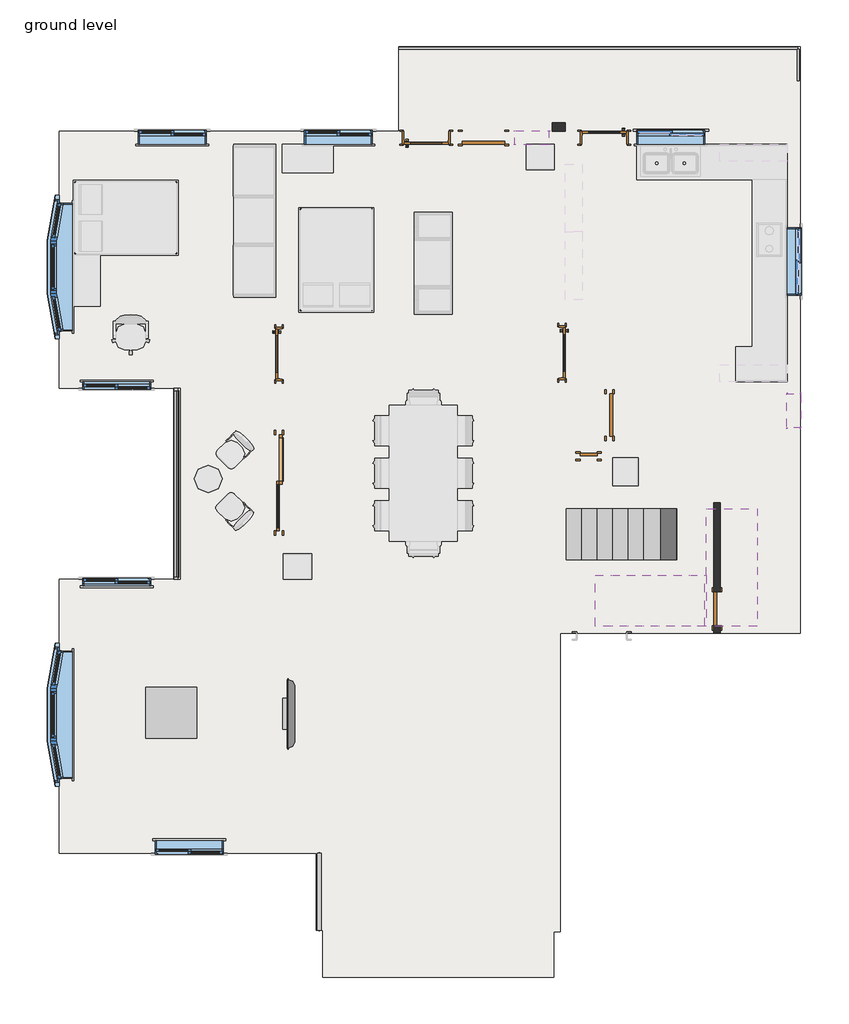
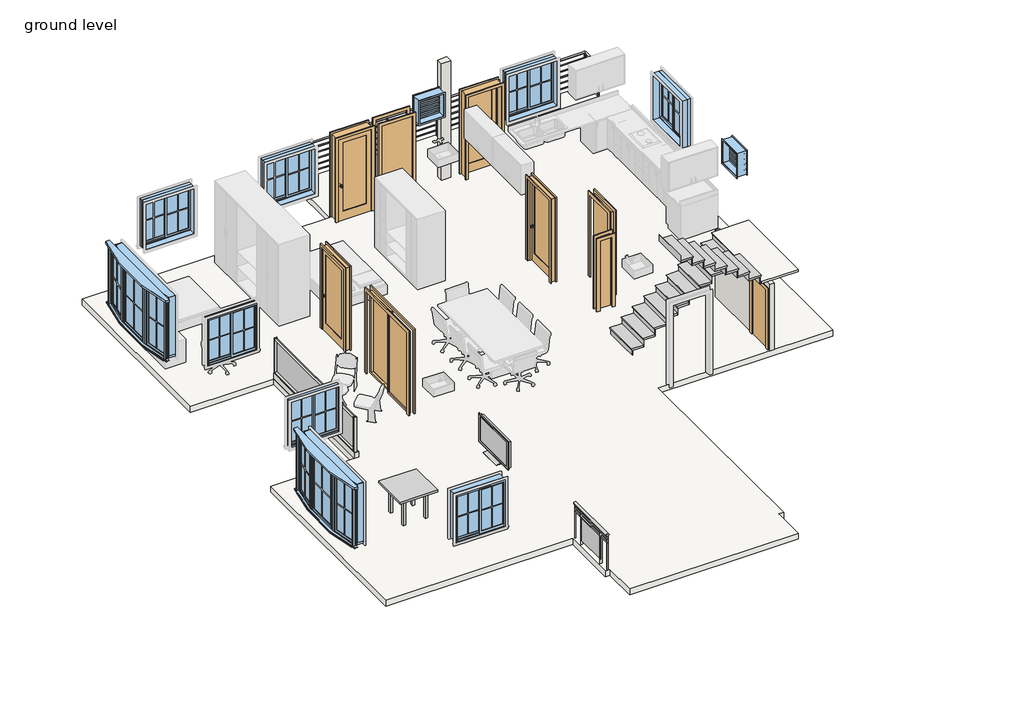
# One storey, part 1 of 2: 11 windows, 9 doors, 4 members, 3 railings, 3 walls, 2 furniture elements, 2 slabs, 2 stair flights, 1 plate.
"""IFC4 building model written with IfcOpenShell, lengths in millimetres."""

from ifc_helpers import new_model, si_unit, point, frame, frame_2d, origin, place, context, project, spatial, polyline, circle_curve, ellipse_curve, trimmed, segment, composite_curve, outline, extrude, transform, mapped, element, save
from ifc_brep_helpers import plane_surface, extruded_surface, advanced_brep
from components import door_505787c2, door_2631f38c, door_a3feeac7, door_3c6ab76a, door_b768bedd, door_bffbd567, door_78caadf7, door_bb98abfd, furniture_0b81fedb, furniture_5106913f, member_e759e848, member_235ee26f, member_c5b617ba, system_panel_glazed_59f99603, non_monolithic_landing_900e45c4, stair_flight_cfa64765, stair_flight_9d522be5, window_bf21e6cb, window_f2d8fef0, window_5af5dca6, window_ba0d9a6f

model = new_model("IFC4")

# Units and contexts
model_context = context("Model", 3, world=origin())
ifc_project = project(units=[si_unit("LENGTHUNIT", "METRE", prefix="MILLI")], contexts=[model_context])

# Site, building, storey
site = spatial("IfcSite", under=ifc_project)
building = spatial("IfcBuilding", under=site)
storey = spatial("IfcBuildingStorey", under=building, Name="ground level", Elevation=609.6)

# Doors
placement = place(None, origin())
door_shape = door_505787c2(model_context)
element("IfcDoor", 1, ObjectType="Door-Double-Sliding : 68\" x 84\"", at=placement, inside=storey, context=model_context, shape_type="MappedRepresentation", body=[
    mapped(door_shape, transform((-10169.8219122, 4291.3668074, 609.6), x_axis=(0.0, -1.0, 0.0), y_axis=(1.0, 0.0, 0.0), z_axis=(0.0, 0.0, 1.0))),
])
door_2_shape = door_2631f38c(model_context)
element("IfcDoor", 2, ObjectType="Door-Interior-Single-1_Panel-Wood : 32\" x 84\"", at=placement, inside=storey, context=model_context, shape_type="MappedRepresentation", body=[
    mapped(door_2_shape, transform((-7401.2219122, 10479.4418074, 609.6), x_axis=(1.0, 0.0, 0.0), y_axis=(0.0, 1.0, 0.0), z_axis=(0.0, 0.0, 1.0))),
])
element("IfcDoor", 3, ObjectType="Door-Interior-Single-1_Panel-Wood : 32\" x 84\"", at=placement, inside=storey, context=model_context, shape_type="MappedRepresentation", body=[
    mapped(door_2_shape, transform((-4203.9969122, 10485.7918074, 609.6), x_axis=(-1.0, 0.0, 0.0), y_axis=(0.0, -1.0, 0.0), z_axis=(0.0, 0.0, 1.0))),
])
door_3_shape = door_a3feeac7(model_context)
element("IfcDoor", 4, ObjectType="Door-Interior-Single-1_Panel-Wood : 36\" x 84\"", at=placement, inside=storey, context=model_context, shape_type="MappedRepresentation", body=[
    mapped(door_3_shape, transform((-10045.9969122, 6602.7668074, 609.6), x_axis=(0.0, -1.0, 0.0), y_axis=(1.0, 0.0, 0.0), z_axis=(0.0, 0.0, 1.0))),
])
door_4_shape = door_3c6ab76a(model_context)
element("IfcDoor", 5, ObjectType="Door-Interior-Single-1_Panel-Wood : 36\" x 84\"", at=placement, inside=storey, context=model_context, shape_type="MappedRepresentation", body=[
    mapped(door_4_shape, transform((-4962.8219122, 6624.9918074, 609.6), x_axis=(0.0, -1.0, 0.0), y_axis=(1.0, 0.0, 0.0), z_axis=(0.0, 0.0, 1.0))),
])
door_5_shape = door_b768bedd(model_context)
element("IfcDoor", 6, ObjectType="Single-Flush : 12\" x 72\"", at=placement, inside=storey, context=model_context, shape_type="MappedRepresentation", body=[
    mapped(door_5_shape, transform((-4486.5719122, 4767.6168074, 609.6), x_axis=(1.0, 0.0, 0.0), y_axis=(0.0, 1.0, 0.0), z_axis=(0.0, 0.0, 1.0))),
])
door_6_shape = door_bffbd567(model_context)
element("IfcDoor", 7, ObjectType="Single-Flush : 24\" x 60\"", at=placement, inside=storey, context=model_context, shape_type="MappedRepresentation", body=[
    mapped(door_6_shape, transform((-2180.7281622, 2027.5918074, 609.6), x_axis=(0.0, -1.0, 0.0), y_axis=(1.0, 0.0, 0.0), z_axis=(0.0, 0.0, 1.0))),
])
door_7_shape = door_78caadf7(model_context)
element("IfcDoor", 8, ObjectType="Single-Flush : 30\" x 84\"", at=placement, inside=storey, context=model_context, shape_type="MappedRepresentation", body=[
    mapped(door_7_shape, transform((-4111.9219122, 5504.2168074, 609.6), x_axis=(0.0, 1.0, 0.0), y_axis=(-1.0, 0.0, 0.0), z_axis=(0.0, 0.0, 1.0))),
])
door_8_shape = door_bb98abfd(model_context)
element("IfcDoor", 9, ObjectType="Single-Flush : 30\" x 84\"", at=placement, inside=storey, context=model_context, shape_type="MappedRepresentation", body=[
    mapped(door_8_shape, transform((-6372.5219122, 10482.6168074, 609.6), x_axis=(-1.0, 0.0, 0.0), y_axis=(0.0, -1.0, 0.0), z_axis=(0.0, 0.0, 1.0))),
])

# Furniture
furniture_shape = furniture_0b81fedb(model_context)
element("IfcFurniture", 10, ObjectType="TV - Flat Screen : 50\" 2", at=placement, inside=storey, context=model_context, shape_type="MappedRepresentation", body=[
    mapped(furniture_shape, transform((-9821.374617, 140.8722933, 1371.6), x_axis=(0.0, -1.0, 0.0), y_axis=(1.0, 0.0, 0.0), z_axis=(0.0, 0.0, 1.0))),
])
furniture_2_shape = furniture_5106913f(model_context)
element("IfcFurniture", 11, ObjectType="Table-Rectangular : 36\" x 36\"", at=placement, inside=storey, context=model_context, shape_type="MappedRepresentation", body=[
    mapped(furniture_2_shape, transform((-11973.2219122, 167.0418074, 609.6), x_axis=(1.0, 0.0, 0.0), y_axis=(0.0, 1.0, 0.0), z_axis=(0.0, 0.0, 1.0))),
])

# Members
member_shape = member_e759e848(model_context)
element("IfcMember", 12, ObjectType="Circular Mullion : 2.5\" Circular", at=placement, inside=storey, context=model_context, shape_type="MappedRepresentation", body=[
    mapped(member_shape, transform((-11890.6719122, 2595.9168074, 1676.4), x_axis=(0.0, 0.0, 1.0), y_axis=(-1.0, 0.0, 0.0), z_axis=(0.0, -1.0, 0.0))),
])
member_2_shape = member_235ee26f(model_context)
element("IfcMember", 13, ObjectType="Rectangular Mullion : 1.5\" x 2.5\" rectangular", at=placement, inside=storey, context=model_context, shape_type="MappedRepresentation", body=[
    mapped(member_2_shape, transform((-11890.6719122, 5947.562262, 762.0), x_axis=(0.0, 0.0, -1.0), y_axis=(-1.0, 0.0, 0.0), z_axis=(0.0, 1.0, 0.0))),
])
member_3_shape = member_c5b617ba(model_context)
element("IfcMember", 14, ObjectType="Rectangular Mullion : 1.5\" x 2.5\" rectangular", at=placement, inside=storey, context=model_context, shape_type="MappedRepresentation", body=[
    mapped(member_3_shape, transform((-11890.6719122, 5985.662262, 1676.4), x_axis=(0.0, 1.0, 0.0), y_axis=(-1.0, 0.0, 0.0), z_axis=(0.0, 0.0, 1.0))),
])
element("IfcMember", 15, ObjectType="Rectangular Mullion : 1.5\" x 2.5\" rectangular", at=placement, inside=storey, context=model_context, shape_type="MappedRepresentation", body=[
    mapped(member_3_shape, transform((-11890.6719122, 2557.8168074, 762.0), x_axis=(0.0, -1.0, 0.0), y_axis=(-1.0, 0.0, 0.0), z_axis=(0.0, 0.0, -1.0))),
])

# Plate
system_panel_glazed_shape = system_panel_glazed_59f99603(model_context)
element("IfcPlate", 16, ObjectType="System Panel : Glazed", at=placement, inside=storey, context=model_context, shape_type="MappedRepresentation", body=[
    mapped(system_panel_glazed_shape, transform((-11890.6719122, 4271.7395347, 800.1), x_axis=(0.0, -1.0, 0.0), y_axis=(1.0, 0.0, 0.0), z_axis=(0.0, 0.0, 1.0))),
])

# Railings
element("IfcRailing", 17, ObjectType="Glass Panel - Bottom Fill", at=placement, inside=storey, context=model_context, shape_type="SolidModel", body=[
    advanced_brep(
    [(-9357.0219122, -3741.3831926, 1524.0), (-9280.8219122, -3741.3831926, 1524.0), (-9357.0219122, -2357.0831926, 1524.0), (-9280.8219122, -2357.0831926, 1524.0)],
    [
        (0, 1, ellipse_curve(frame((-9318.9219122, -3741.3831926, 1524.0), z_axis=(0.0, -1.0, 0.0), x_axis=(1.0, 0.0, 0.0)), 38.1, 28.575)),
        (1, 0, ellipse_curve(frame((-9318.9219122, -3741.3831926, 1524.0), z_axis=(0.0, -1.0, 0.0), x_axis=(1.0, 0.0, 0.0)), 38.1, 28.575)),
        (2, 3, ellipse_curve(frame((-9318.9219122, -2357.0831926, 1524.0), z_axis=(0.0, 1.0, 0.0), x_axis=(1.0, 0.0, 0.0)), 38.1, 28.575)),
        (3, 2, ellipse_curve(frame((-9318.9219122, -2357.0831926, 1524.0), z_axis=(0.0, 1.0, 0.0), x_axis=(1.0, 0.0, 0.0)), 38.1, 28.575)),
        (0, 2),
        (3, 1),
    ],
    [
        plane_surface(frame((-9318.9219122, -3741.3831926, 1524.0), z_axis=(0.0, -1.0, 0.0), x_axis=(0.0, 0.0, 1.0))),
        plane_surface(frame((-9318.9219122, -2357.0831926, 1524.0), z_axis=(0.0, 1.0, 0.0), x_axis=(0.0, 0.0, 1.0))),
        extruded_surface(trimmed(ellipse_curve(frame((-9318.9219122, -2357.0831926, 1524.0), z_axis=(0.0, -1.0, 0.0), x_axis=(1.0, 0.0, 0.0)), 38.1, 28.575), [point((-9357.0219122, -2357.0831926, 1524.0))], [point((-9280.8219122, -2357.0831926, 1524.0))], True, "CARTESIAN"), (0.0, -1384.2999999999997, 0.0), 1384.2999999999997),
        extruded_surface(trimmed(ellipse_curve(frame((-9318.9219122, -2357.0831926, 1524.0), z_axis=(0.0, -1.0, 0.0), x_axis=(1.0, 0.0, 0.0)), 38.1, 28.575), [point((-9280.8219122, -2357.0831926, 1524.0))], [point((-9357.0219122, -2357.0831926, 1524.0))], True, "CARTESIAN"), (0.0, -1384.2999999999997, 0.0), 1384.2999999999997),
    ],
    [
        (0, [[1, 2]]),
        (1, [[3, 4]]),
        (2, [[-1, 5, -4, 6]]),
        (3, [[-2, -6, -3, -5]]),
    ],
),
    extrude(outline(polyline([(-9306.2219122, -3741.3831926), (-9331.6219122, -3741.3831926), (-9331.6219122, -2357.0831926), (-9306.2219122, -2357.0831926), (-9306.2219122, -3741.3831926)])), frame((0.0, 0.0, 1409.7), z_axis=(0.0, 0.0, 1.0), x_axis=(1.0, 0.0, 0.0)), (0.0, 0.0, 1.0), 25.4),
    extrude(outline(polyline([(-9306.2219122, -3741.3831926), (-9331.6219122, -3741.3831926), (-9331.6219122, -2357.0831926), (-9306.2219122, -2357.0831926), (-9306.2219122, -3741.3831926)])), frame((0.0, 0.0, 1308.1), z_axis=(0.0, 0.0, 1.0), x_axis=(1.0, 0.0, 0.0)), (0.0, 0.0, 1.0), 25.4),
    extrude(outline(polyline([(-9293.5219122, -2649.1831926), (-9344.3219122, -2649.1831926), (-9344.3219122, -2636.4831926), (-9293.5219122, -2636.4831926), (-9293.5219122, -2649.1831926)])), frame((0.0, 0.0, 609.6), z_axis=(0.0, 0.0, 1.0), x_axis=(1.0, 0.0, 0.0)), (0.0, 0.0, 1.0), 885.825),
    extrude(outline(polyline([(-9325.4570692, -3455.6331926), (-9325.4570692, -2642.8331926), (-9319.1070692, -2642.8331926), (-9319.1070692, -3455.6331926), (-9325.4570692, -3455.6331926)])), frame((0.0, 0.0, 711.2), z_axis=(0.0, 0.0, 1.0), x_axis=(1.0, 0.0, 0.0)), (0.0, 0.0, 1.0), 596.9),
    extrude(outline(polyline([(-9293.5219122, -3461.9831926), (-9344.3219122, -3461.9831926), (-9344.3219122, -3449.2831926), (-9293.5219122, -3449.2831926), (-9293.5219122, -3461.9831926)])), frame((0.0, 0.0, 609.6), z_axis=(0.0, 0.0, 1.0), x_axis=(1.0, 0.0, 0.0)), (0.0, 0.0, 1.0), 885.825),
    extrude(outline(polyline([(-9309.3969122, -2369.7831926), (-9328.4469122, -2369.7831926), (-9328.4469122, -2350.7331926), (-9309.3969122, -2350.7331926), (-9309.3969122, -2369.7831926)])), frame((0.0, 0.0, 609.6), z_axis=(0.0, 0.0, 1.0), x_axis=(1.0, 0.0, 0.0)), (0.0, 0.0, 1.0), 885.825),
    extrude(outline(polyline([(-9309.3969122, -3747.7331926), (-9328.4469122, -3747.7331926), (-9328.4469122, -3728.6831926), (-9309.3969122, -3728.6831926), (-9309.3969122, -3747.7331926)])), frame((0.0, 0.0, 609.6), z_axis=(0.0, 0.0, 1.0), x_axis=(1.0, 0.0, 0.0)), (0.0, 0.0, 1.0), 885.825),
])
element("IfcRailing", 18, ObjectType="Handrail - Pipe", at=placement, inside=storey, context=model_context, shape_type="SweptSolid", body=[
    extrude(outline(composite_curve([segment(trimmed(circle_curve(frame_2d((1504.95, -727.3719122)), 19.05), [point((1504.95, -708.3219122))], [point((1504.95, -746.4219122))], False, "CARTESIAN"), True, "CONTINUOUS"), segment(trimmed(circle_curve(frame_2d((1504.95, -727.3719122)), 19.05), [point((1504.95, -746.4219122))], [point((1504.95, -708.3219122))], False, "CARTESIAN"), True, "CONTINUOUS")], self_intersect=False)), frame((0.0, 11511.3168074, 0.0), z_axis=(0.0, 1.0, 0.0), x_axis=(0.0, 0.0, 1.0)), (0.0, 0.0, 1.0), 558.8),
    extrude(outline(composite_curve([segment(trimmed(circle_curve(frame_2d((1358.9, -727.3719122)), 12.7), [point((1358.9, -740.0719122))], [point((1358.9, -714.6719122))], False, "CARTESIAN"), True, "CONTINUOUS"), segment(trimmed(circle_curve(frame_2d((1358.9, -727.3719122)), 12.7), [point((1358.9, -714.6719122))], [point((1358.9, -740.0719122))], False, "CARTESIAN"), True, "CONTINUOUS")], self_intersect=False)), frame((0.0, 11511.3168074, 0.0), z_axis=(0.0, 1.0, 0.0), x_axis=(0.0, 0.0, 1.0)), (0.0, 0.0, 1.0), 558.8),
    extrude(outline(composite_curve([segment(trimmed(circle_curve(frame_2d((1206.5, -727.3719122)), 12.7), [point((1206.5, -740.0719122))], [point((1206.5, -714.6719122))], False, "CARTESIAN"), True, "CONTINUOUS"), segment(trimmed(circle_curve(frame_2d((1206.5, -727.3719122)), 12.7), [point((1206.5, -714.6719122))], [point((1206.5, -740.0719122))], False, "CARTESIAN"), True, "CONTINUOUS")], self_intersect=False)), frame((0.0, 11511.3168074, 0.0), z_axis=(0.0, 1.0, 0.0), x_axis=(0.0, 0.0, 1.0)), (0.0, 0.0, 1.0), 558.8),
    extrude(outline(composite_curve([segment(trimmed(circle_curve(frame_2d((1054.1, -727.3719122)), 12.7), [point((1054.1, -740.0719122))], [point((1054.1, -714.6719122))], False, "CARTESIAN"), True, "CONTINUOUS"), segment(trimmed(circle_curve(frame_2d((1054.1, -727.3719122)), 12.7), [point((1054.1, -714.6719122))], [point((1054.1, -740.0719122))], False, "CARTESIAN"), True, "CONTINUOUS")], self_intersect=False)), frame((0.0, 11511.3168074, 0.0), z_axis=(0.0, 1.0, 0.0), x_axis=(0.0, 0.0, 1.0)), (0.0, 0.0, 1.0), 558.8),
    extrude(outline(composite_curve([segment(trimmed(circle_curve(frame_2d((901.7, -727.3719122)), 12.7), [point((901.7, -740.0719122))], [point((901.7, -714.6719122))], False, "CARTESIAN"), True, "CONTINUOUS"), segment(trimmed(circle_curve(frame_2d((901.7, -727.3719122)), 12.7), [point((901.7, -714.6719122))], [point((901.7, -740.0719122))], False, "CARTESIAN"), True, "CONTINUOUS")], self_intersect=False)), frame((0.0, 11511.3168074, 0.0), z_axis=(0.0, 1.0, 0.0), x_axis=(0.0, 0.0, 1.0)), (0.0, 0.0, 1.0), 558.8),
    extrude(outline(composite_curve([segment(trimmed(circle_curve(frame_2d((749.3, -727.3719122)), 12.7), [point((749.3, -740.0719122))], [point((749.3, -714.6719122))], False, "CARTESIAN"), True, "CONTINUOUS"), segment(trimmed(circle_curve(frame_2d((749.3, -727.3719122)), 12.7), [point((749.3, -714.6719122))], [point((749.3, -740.0719122))], False, "CARTESIAN"), True, "CONTINUOUS")], self_intersect=False)), frame((0.0, 11511.3168074, 0.0), z_axis=(0.0, 1.0, 0.0), x_axis=(0.0, 0.0, 1.0)), (0.0, 0.0, 1.0), 558.8),
    extrude(outline(composite_curve([segment(trimmed(circle_curve(frame_2d((-727.3719122, 12057.4168074)), 12.7), [point((-740.0719122, 12057.4168074))], [point((-714.6719122, 12057.4168074))], False, "CARTESIAN"), True, "CONTINUOUS"), segment(trimmed(circle_curve(frame_2d((-727.3719122, 12057.4168074)), 12.7), [point((-714.6719122, 12057.4168074))], [point((-740.0719122, 12057.4168074))], False, "CARTESIAN"), True, "CONTINUOUS")], self_intersect=False)), frame((0.0, 0.0, 609.6), z_axis=(0.0, 0.0, 1.0), x_axis=(1.0, 0.0, 0.0)), (0.0, 0.0, 1.0), 876.3),
    extrude(outline(composite_curve([segment(trimmed(circle_curve(frame_2d((-727.3719122, 11524.0168074)), 12.7), [point((-740.0719122, 11524.0168074))], [point((-714.6719122, 11524.0168074))], False, "CARTESIAN"), True, "CONTINUOUS"), segment(trimmed(circle_curve(frame_2d((-727.3719122, 11524.0168074)), 12.7), [point((-714.6719122, 11524.0168074))], [point((-740.0719122, 11524.0168074))], False, "CARTESIAN"), True, "CONTINUOUS")], self_intersect=False)), frame((0.0, 0.0, 609.6), z_axis=(0.0, 0.0, 1.0), x_axis=(1.0, 0.0, 0.0)), (0.0, 0.0, 1.0), 876.3),
])
element("IfcRailing", 19, ObjectType="Handrail - Pipe", at=placement, inside=storey, context=model_context, shape_type="SweptSolid", body=[
    extrude(outline(composite_curve([segment(trimmed(circle_curve(frame_2d((12090.8688347, 1504.95)), 19.05), [point((12109.9188347, 1504.95))], [point((12071.8188347, 1504.95))], False, "CARTESIAN"), True, "CONTINUOUS"), segment(trimmed(circle_curve(frame_2d((12090.8688347, 1504.95)), 19.05), [point((12071.8188347, 1504.95))], [point((12109.9188347, 1504.95))], False, "CARTESIAN"), True, "CONTINUOUS")], self_intersect=False)), frame((-7890.1719122, 0.0, 0.0), z_axis=(1.0, 0.0, 0.0), x_axis=(0.0, 1.0, 0.0)), (0.0, 0.0, 1.0), 7160.6305666),
    extrude(outline(composite_curve([segment(trimmed(circle_curve(frame_2d((12090.8688347, 1358.9)), 12.7), [point((12078.1688347, 1358.9))], [point((12103.5688347, 1358.9))], False, "CARTESIAN"), True, "CONTINUOUS"), segment(trimmed(circle_curve(frame_2d((12090.8688347, 1358.9)), 12.7), [point((12103.5688347, 1358.9))], [point((12078.1688347, 1358.9))], False, "CARTESIAN"), True, "CONTINUOUS")], self_intersect=False)), frame((-7890.1719122, 0.0, 0.0), z_axis=(1.0, 0.0, 0.0), x_axis=(0.0, 1.0, 0.0)), (0.0, 0.0, 1.0), 7160.6305666),
    extrude(outline(composite_curve([segment(trimmed(circle_curve(frame_2d((12090.8688347, 1206.5)), 12.7), [point((12078.1688347, 1206.5))], [point((12103.5688347, 1206.5))], False, "CARTESIAN"), True, "CONTINUOUS"), segment(trimmed(circle_curve(frame_2d((12090.8688347, 1206.5)), 12.7), [point((12103.5688347, 1206.5))], [point((12078.1688347, 1206.5))], False, "CARTESIAN"), True, "CONTINUOUS")], self_intersect=False)), frame((-7890.1719122, 0.0, 0.0), z_axis=(1.0, 0.0, 0.0), x_axis=(0.0, 1.0, 0.0)), (0.0, 0.0, 1.0), 7160.6305666),
    extrude(outline(composite_curve([segment(trimmed(circle_curve(frame_2d((12090.8688347, 1054.1)), 12.7), [point((12078.1688347, 1054.1))], [point((12103.5688347, 1054.1))], False, "CARTESIAN"), True, "CONTINUOUS"), segment(trimmed(circle_curve(frame_2d((12090.8688347, 1054.1)), 12.7), [point((12103.5688347, 1054.1))], [point((12078.1688347, 1054.1))], False, "CARTESIAN"), True, "CONTINUOUS")], self_intersect=False)), frame((-7890.1719122, 0.0, 0.0), z_axis=(1.0, 0.0, 0.0), x_axis=(0.0, 1.0, 0.0)), (0.0, 0.0, 1.0), 7160.6305666),
    extrude(outline(composite_curve([segment(trimmed(circle_curve(frame_2d((12090.8688347, 901.7)), 12.7), [point((12078.1688347, 901.7))], [point((12103.5688347, 901.7))], False, "CARTESIAN"), True, "CONTINUOUS"), segment(trimmed(circle_curve(frame_2d((12090.8688347, 901.7)), 12.7), [point((12103.5688347, 901.7))], [point((12078.1688347, 901.7))], False, "CARTESIAN"), True, "CONTINUOUS")], self_intersect=False)), frame((-7890.1719122, 0.0, 0.0), z_axis=(1.0, 0.0, 0.0), x_axis=(0.0, 1.0, 0.0)), (0.0, 0.0, 1.0), 7160.6305666),
    extrude(outline(composite_curve([segment(trimmed(circle_curve(frame_2d((12090.8688347, 749.3)), 12.7), [point((12078.1688347, 749.3))], [point((12103.5688347, 749.3))], False, "CARTESIAN"), True, "CONTINUOUS"), segment(trimmed(circle_curve(frame_2d((12090.8688347, 749.3)), 12.7), [point((12103.5688347, 749.3))], [point((12078.1688347, 749.3))], False, "CARTESIAN"), True, "CONTINUOUS")], self_intersect=False)), frame((-7890.1719122, 0.0, 0.0), z_axis=(1.0, 0.0, 0.0), x_axis=(0.0, 1.0, 0.0)), (0.0, 0.0, 1.0), 7160.6305666),
    extrude(outline(composite_curve([segment(trimmed(circle_curve(frame_2d((-6825.5413455, 12090.8688347)), 12.7), [point((-6825.5413455, 12078.1688347))], [point((-6825.5413455, 12103.5688347))], False, "CARTESIAN"), True, "CONTINUOUS"), segment(trimmed(circle_curve(frame_2d((-6825.5413455, 12090.8688347)), 12.7), [point((-6825.5413455, 12103.5688347))], [point((-6825.5413455, 12078.1688347))], False, "CARTESIAN"), True, "CONTINUOUS")], self_intersect=False)), frame((0.0, 0.0, 609.6), z_axis=(0.0, 0.0, 1.0), x_axis=(1.0, 0.0, 0.0)), (0.0, 0.0, 1.0), 876.3),
    extrude(outline(composite_curve([segment(trimmed(circle_curve(frame_2d((-5606.3413455, 12090.8688347)), 12.7), [point((-5606.3413455, 12078.1688347))], [point((-5606.3413455, 12103.5688347))], False, "CARTESIAN"), True, "CONTINUOUS"), segment(trimmed(circle_curve(frame_2d((-5606.3413455, 12090.8688347)), 12.7), [point((-5606.3413455, 12103.5688347))], [point((-5606.3413455, 12078.1688347))], False, "CARTESIAN"), True, "CONTINUOUS")], self_intersect=False)), frame((0.0, 0.0, 609.6), z_axis=(0.0, 0.0, 1.0), x_axis=(1.0, 0.0, 0.0)), (0.0, 0.0, 1.0), 876.3),
    extrude(outline(composite_curve([segment(trimmed(circle_curve(frame_2d((-4387.1413455, 12090.8688347)), 12.7), [point((-4387.1413455, 12078.1688347))], [point((-4387.1413455, 12103.5688347))], False, "CARTESIAN"), True, "CONTINUOUS"), segment(trimmed(circle_curve(frame_2d((-4387.1413455, 12090.8688347)), 12.7), [point((-4387.1413455, 12103.5688347))], [point((-4387.1413455, 12078.1688347))], False, "CARTESIAN"), True, "CONTINUOUS")], self_intersect=False)), frame((0.0, 0.0, 609.6), z_axis=(0.0, 0.0, 1.0), x_axis=(1.0, 0.0, 0.0)), (0.0, 0.0, 1.0), 876.3),
    extrude(outline(composite_curve([segment(trimmed(circle_curve(frame_2d((-3167.9413455, 12090.8688347)), 12.7), [point((-3167.9413455, 12078.1688347))], [point((-3167.9413455, 12103.5688347))], False, "CARTESIAN"), True, "CONTINUOUS"), segment(trimmed(circle_curve(frame_2d((-3167.9413455, 12090.8688347)), 12.7), [point((-3167.9413455, 12103.5688347))], [point((-3167.9413455, 12078.1688347))], False, "CARTESIAN"), True, "CONTINUOUS")], self_intersect=False)), frame((0.0, 0.0, 609.6), z_axis=(0.0, 0.0, 1.0), x_axis=(1.0, 0.0, 0.0)), (0.0, 0.0, 1.0), 876.3),
    extrude(outline(composite_curve([segment(trimmed(circle_curve(frame_2d((-1948.7413455, 12090.8688347)), 12.7), [point((-1948.7413455, 12078.1688347))], [point((-1948.7413455, 12103.5688347))], False, "CARTESIAN"), True, "CONTINUOUS"), segment(trimmed(circle_curve(frame_2d((-1948.7413455, 12090.8688347)), 12.7), [point((-1948.7413455, 12103.5688347))], [point((-1948.7413455, 12078.1688347))], False, "CARTESIAN"), True, "CONTINUOUS")], self_intersect=False)), frame((0.0, 0.0, 609.6), z_axis=(0.0, 0.0, 1.0), x_axis=(1.0, 0.0, 0.0)), (0.0, 0.0, 1.0), 876.3),
    extrude(outline(composite_curve([segment(trimmed(circle_curve(frame_2d((-7877.4719122, 12090.8688347)), 12.7), [point((-7877.4719122, 12078.1688347))], [point((-7877.4719122, 12103.5688347))], False, "CARTESIAN"), True, "CONTINUOUS"), segment(trimmed(circle_curve(frame_2d((-7877.4719122, 12090.8688347)), 12.7), [point((-7877.4719122, 12103.5688347))], [point((-7877.4719122, 12078.1688347))], False, "CARTESIAN"), True, "CONTINUOUS")], self_intersect=False)), frame((0.0, 0.0, 609.6), z_axis=(0.0, 0.0, 1.0), x_axis=(1.0, 0.0, 0.0)), (0.0, 0.0, 1.0), 876.3),
    extrude(outline(composite_curve([segment(trimmed(circle_curve(frame_2d((-742.2413455, 12090.8688347)), 12.7), [point((-742.2413455, 12078.1688347))], [point((-742.2413455, 12103.5688347))], False, "CARTESIAN"), True, "CONTINUOUS"), segment(trimmed(circle_curve(frame_2d((-742.2413455, 12090.8688347)), 12.7), [point((-742.2413455, 12103.5688347))], [point((-742.2413455, 12078.1688347))], False, "CARTESIAN"), True, "CONTINUOUS")], self_intersect=False)), frame((0.0, 0.0, 609.6), z_axis=(0.0, 0.0, 1.0), x_axis=(1.0, 0.0, 0.0)), (0.0, 0.0, 1.0), 876.3),
])

# Slabs
element("IfcSlab", 20, ObjectType="Generic - 6\"", at=placement, inside=storey, context=model_context, shape_type="SweptSolid", body=[
    extrude(outline(polyline([(-7890.1719122, 10596.9168074), (-7890.1719122, 12120.9168074), (-689.2719122, 12120.9168074), (-689.2719122, 1595.7918074), (-4994.5719122, 1595.7918074), (-4994.5719122, -2357.0831926), (-4993.7781622, -2357.0831926), (-4993.7781622, -3766.7831926), (-5108.0781622, -3766.7831926), (-5108.0781622, -4585.9331926), (-9261.7719122, -4585.9331926), (-9261.7719122, -3741.3831926), (-9376.0719122, -3741.3831926), (-9376.0719122, -2357.0831926), (-13986.1719122, -2357.0831926), (-13986.1719122, 2557.8168074), (-11928.7719122, 2557.8168074), (-11928.7719122, 5985.662262), (-13986.1719122, 5985.662262), (-13986.1719122, 10596.9168074), (-7890.1719122, 10596.9168074)])), frame((0.0, 0.0, 457.2), z_axis=(0.0, 0.0, 1.0), x_axis=(1.0, 0.0, 0.0)), (0.0, 0.0, 1.0), 152.4),
])
non_monolithic_landing_shape = non_monolithic_landing_900e45c4(model_context)
element("IfcSlab", 21, ObjectType="Non-Monolithic Landing", at=placement, inside=storey, context=model_context, shape_type="MappedRepresentation", body=[
    mapped(non_monolithic_landing_shape, transform((0.0, 0.0, 0.0), x_axis=(1.0, 0.0, 0.0), y_axis=(0.0, 1.0, 0.0), z_axis=(0.0, 0.0, 1.0))),
])

# Stair flights
stair_flight_shape = stair_flight_cfa64765(model_context)
element("IfcStairFlight", 22, ObjectType="2\" Tread 1\" Nosing 1/4\" Riser", at=placement, inside=storey, context=model_context, shape_type="MappedRepresentation", body=[
    mapped(stair_flight_shape, transform((0.0, 0.0, 0.0), x_axis=(1.0, 0.0, 0.0), y_axis=(0.0, 1.0, 0.0), z_axis=(0.0, 0.0, 1.0))),
])
stair_flight_2_shape = stair_flight_9d522be5(model_context)
element("IfcStairFlight", 23, ObjectType="2\" Tread 1\" Nosing 1/4\" Riser", at=placement, inside=storey, context=model_context, shape_type="MappedRepresentation", body=[
    mapped(stair_flight_2_shape, transform((0.0, 0.0, 0.0), x_axis=(1.0, 0.0, 0.0), y_axis=(0.0, 1.0, 0.0), z_axis=(0.0, 0.0, 1.0))),
])

# Walls
element("IfcWall", 24, ObjectType="Generic - 4.5\"", at=placement, inside=storey, context=model_context, shape_type="SweptSolid", body=[
    extrude(outline(polyline([(1722.7918074, 2133.6), (1722.7918074, 609.6), (1595.7918074, 609.6), (1595.7918074, 2336.8), (3929.4168074, 2336.8), (3929.4168074, 609.6), (2332.3918074, 609.6), (2332.3918074, 2133.6), (1722.7918074, 2133.6)])), frame((-2237.8781622, 0.0, 0.0), z_axis=(1.0, 0.0, 0.0), x_axis=(0.0, 1.0, 0.0)), (0.0, 0.0, 1.0), 114.3),
])
element("IfcWall", 25, ObjectType="Generic - 4.5\"", at=placement, inside=storey, context=model_context, shape_type="SweptSolid", body=[
    extrude(outline(polyline([(-11928.7719122, 2557.8168074), (-11928.7719122, 5985.662262), (-11814.4719122, 5985.662262), (-11814.4719122, 2557.8168074), (-11928.7719122, 2557.8168074)])), frame((0.0, 0.0, 609.6), z_axis=(0.0, 0.0, 1.0), x_axis=(1.0, 0.0, 0.0)), (0.0, 0.0, 1.0), 152.4),
])
element("IfcWall", 26, ObjectType="Generic - 9\"", at=placement, inside=storey, context=model_context, shape_type="SweptSolid", body=[
    extrude(outline(polyline([(-4908.8469122, 10749.3168074), (-4908.8469122, 10596.9168074), (-5137.4469122, 10596.9168074), (-5137.4469122, 10749.3168074), (-4908.8469122, 10749.3168074)])), frame((0.0, 0.0, 609.6), z_axis=(0.0, 0.0, 1.0), x_axis=(1.0, 0.0, 0.0)), (0.0, 0.0, 1.0), 3048.0),
])

# Windows
window_shape = window_bf21e6cb(model_context)
element("IfcWindow", 27, ObjectType="Window-Bay-Casement-10_Degree_Angle : 90\" x 60\" x 6\"", at=placement, inside=storey, context=model_context, shape_type="MappedRepresentation", body=[
    mapped(window_shape, transform((-13871.8719122, 8161.6918074, 609.6), x_axis=(0.0, 1.0, 0.0), y_axis=(-1.0, 0.0, 0.0), z_axis=(0.0, 0.0, 1.0))),
])
element("IfcWindow", 28, ObjectType="Window-Bay-Casement-10_Degree_Angle : 90\" x 60\" x 6\"", at=placement, inside=storey, context=model_context, shape_type="MappedRepresentation", body=[
    mapped(window_shape, transform((-13871.8719122, 128.9418074, 609.6), x_axis=(0.0, 1.0, 0.0), y_axis=(-1.0, 0.0, 0.0), z_axis=(0.0, 0.0, 1.0))),
])
window_2_shape = window_f2d8fef0(model_context)
element("IfcWindow", 29, ObjectType="Window-Louvers : 24\" x 24\"", at=placement, inside=storey, context=model_context, shape_type="MappedRepresentation", body=[
    mapped(window_2_shape, transform((-5505.7469122, 10488.9668074, 1524.0), x_axis=(1.0, 0.0, 0.0), y_axis=(0.0, 1.0, 0.0), z_axis=(0.0, 0.0, 1.0))),
])
element("IfcWindow", 30, ObjectType="Window-Louvers : 24\" x 24\"", at=placement, inside=storey, context=model_context, shape_type="MappedRepresentation", body=[
    mapped(window_2_shape, transform((-797.2219122, 5586.7668074, 1524.0), x_axis=(0.0, -1.0, 0.0), y_axis=(1.0, 0.0, 0.0), z_axis=(0.0, 0.0, 1.0))),
])
window_3_shape = window_5af5dca6(model_context)
element("IfcWindow", 31, ObjectType="Window-Sliding-Double : 48\" x 48\"", at=placement, inside=storey, context=model_context, shape_type="MappedRepresentation", body=[
    mapped(window_3_shape, transform((-11652.5469122, -2246.5931926, 609.6), x_axis=(-1.0, 0.0, 0.0), y_axis=(0.0, -1.0, 0.0), z_axis=(0.0, 0.0, 1.0))),
])
element("IfcWindow", 32, ObjectType="Window-Sliding-Double : 48\" x 48\"", at=placement, inside=storey, context=model_context, shape_type="MappedRepresentation", body=[
    mapped(window_3_shape, transform((-799.7619122, 8263.2918074, 838.2), x_axis=(0.0, -1.0, 0.0), y_axis=(1.0, 0.0, 0.0), z_axis=(0.0, 0.0, 1.0))),
])
element("IfcWindow", 33, ObjectType="Window-Sliding-Double : 48\" x 48\"", at=placement, inside=storey, context=model_context, shape_type="MappedRepresentation", body=[
    mapped(window_3_shape, transform((-8976.0219122, 10486.4268074, 609.6), x_axis=(1.0, 0.0, 0.0), y_axis=(0.0, 1.0, 0.0), z_axis=(0.0, 0.0, 1.0))),
])
element("IfcWindow", 34, ObjectType="Window-Sliding-Double : 48\" x 48\"", at=placement, inside=storey, context=model_context, shape_type="MappedRepresentation", body=[
    mapped(window_3_shape, transform((-11957.3469122, 10486.4268074, 609.6), x_axis=(1.0, 0.0, 0.0), y_axis=(0.0, 1.0, 0.0), z_axis=(0.0, 0.0, 1.0))),
])
element("IfcWindow", 35, ObjectType="Window-Sliding-Double : 48\" x 48\"", at=placement, inside=storey, context=model_context, shape_type="MappedRepresentation", body=[
    mapped(window_3_shape, transform((-3010.1969122, 10486.4268074, 812.8), x_axis=(1.0, 0.0, 0.0), y_axis=(0.0, 1.0, 0.0), z_axis=(0.0, 0.0, 1.0))),
])
window_4_shape = window_ba0d9a6f(model_context)
element("IfcWindow", 36, ObjectType="Window-Sliding-Double : 48\" x 48\"", at=placement, inside=storey, context=model_context, shape_type="MappedRepresentation", body=[
    mapped(window_4_shape, transform((-12957.4719122, 2504.4768074, 609.6), x_axis=(1.0, 0.0, 0.0), y_axis=(0.0, 1.0, 0.0), z_axis=(0.0, 0.0, 1.0))),
])
element("IfcWindow", 37, ObjectType="Window-Sliding-Double : 48\" x 48\"", at=placement, inside=storey, context=model_context, shape_type="MappedRepresentation", body=[
    mapped(window_4_shape, transform((-12957.4719122, 6040.1568074, 609.6), x_axis=(-1.0, 0.0, 0.0), y_axis=(0.0, -1.0, 0.0), z_axis=(0.0, 0.0, 1.0))),
])

save(model, "model.ifc")

# Revit data of these elements
# Type "Door-Double-Sliding : 68\" x 84\""
#   Type Mark = "12"
#   Construction Type Id = "opn-d45"
#   Assembly Code = "C1020"
#   Analytic Construction = "Wood frame, double glass door "
#   Thickness = 0' - 2"
#   Thermal Resistance (R) = 1.8150 (h·ft²·°F)/BTU
#   Heat Transfer Coefficient (U) = 0.5510 BTU/(h·ft²·°F)
#   Height = 7' - 0"
#   Rail Width = 0' - 2"
#   Stiles = 0' - 2"
#   Trim Projection Ext = 0' - 1"
#   Trim Projection Int = 0' - 1"
#   Trim Width = 0' - 3"
#   Width = 5' - 8"
#   Define Thermal Properties by = 1
#   Glazing = Glass
#   Panel Material = Wood - Birch - Solid Stained Light Low Gloss
#   Trim Material = Paint - Sienna
#   Visual Light Transmittance = 0
#   Solar Heat Gain Coefficient = 0
#   Function = (empty or 0)
#   Wall Closure = (empty or 0)
# Type "Door-Interior-Single-1_Panel-Wood : 32\" x 84\""
#   Type Mark = "9"
#   Assembly Code = "C1020300"
#   Analytic Construction = "Wooden"
#   Top Rail = 0' - 4 11/16"
#   Thickness = 0' - 1 3/8"
#   Thermal Resistance (R) = 2.5876 (h·ft²·°F)/BTU
#   Swing Angle [instance default] = 90.00°
#   Stiles = 0' - 4 3/4"
#   Rough Width = 2' - 10"
#   Rough Height = 7' - 1"
#   Height = 7' - 0"
#   Width = 2' - 8"
#   Heat Transfer Coefficient (U) = 0.3865 BTU/(h·ft²·°F)
#   Bottom Rail = 0' - 9 1/8"
#   Trim Material = Cherry
#   Panel Material = Cherry
#   Frame Material = Cherry
#   Door Handle Material = Aluminum
#   Visual Light Transmittance = 0
#   Solar Heat Gain Coefficient = 0
#   Wall Closure = (empty or 0)
#   Function = (empty or 0)
# Type "Door-Interior-Single-1_Panel-Wood : 36\" x 84\""
#   Type Mark = "8"
#   Assembly Code = "C1020300"
#   Analytic Construction = "Wooden"
#   Top Rail = 0' - 4 11/16"
#   Thickness = 0' - 1 3/8"
#   Thermal Resistance (R) = 2.5876 (h·ft²·°F)/BTU
#   Swing Angle [instance default] = 90.00°
#   Stiles = 0' - 4 3/4"
#   Rough Width = 3' - 2"
#   Rough Height = 7' - 1"
#   Height = 7' - 0"
#   Width = 3' - 0"
#   Heat Transfer Coefficient (U) = 0.3865 BTU/(h·ft²·°F)
#   Bottom Rail = 0' - 9 1/8"
#   Trim Material = Cherry
#   Panel Material = Cherry
#   Frame Material = Cherry
#   Door Handle Material = Aluminum
#   Visual Light Transmittance = 0
#   Solar Heat Gain Coefficient = 0
#   Wall Closure = (empty or 0)
#   Function = (empty or 0)
# Type "Single-Flush : 12\" x 72\""
#   Type Mark = "5"
#   Construction Type Id = "MDOOR"
#   Assembly Code = "C1020"
#   Analytic Construction = "Metal"
#   Thickness = 0' - 2"
#   Heat Transfer Coefficient (U) = 0.651978 BTU/(h·ft²·°F)
#   Height = 6' - 0"
#   Trim Projection Ext = 0' - 1"
#   Trim Projection Int = 0' - 1"
#   Trim Width = 0' - 3"
#   Width = 1' - 0"
#   Define Thermal Properties by = 1
#   Define Thermal Properties by = 1
#   Door Material = Door - Panel
#   Frame Material = Door - Frame
#   Visual Light Transmittance = 0
#   Solar Heat Gain Coefficient = 0
#   Function = (empty or 0)
#   Wall Closure = (empty or 0)
# Type "Single-Flush : 24\" x 60\""
#   Type Mark = "13"
#   Construction Type Id = "MDOOR"
#   Assembly Code = "C1020"
#   Analytic Construction = "Metal"
#   Thickness = 0' - 2"
#   Heat Transfer Coefficient (U) = 0.651978 BTU/(h·ft²·°F)
#   Height = 5' - 0"
#   Trim Projection Ext = 0' - 1"
#   Trim Projection Int = 0' - 1"
#   Trim Width = 0' - 3"
#   Width = 2' - 0"
#   Define Thermal Properties by = 1
#   Door Material = Door - Panel
#   Frame Material = Door - Frame
#   Visual Light Transmittance = 0
#   Solar Heat Gain Coefficient = 0
#   Function = (empty or 0)
#   Wall Closure = (empty or 0)
# Type "Single-Flush : 30\" x 84\""
#   Type Mark = "4"
#   Construction Type Id = "MDOOR"
#   Assembly Code = "C1020"
#   Analytic Construction = "Metal"
#   Thickness = 0' - 2"
#   Heat Transfer Coefficient (U) = 0.651978 BTU/(h·ft²·°F)
#   Height = 7' - 0"
#   Trim Projection Ext = 0' - 1"
#   Trim Projection Int = 0' - 1"
#   Trim Width = 0' - 3"
#   Width = 2' - 6"
#   Define Thermal Properties by = 1
#   Define Thermal Properties by = 1
#   Door Material = Door - Panel
#   Frame Material = Door - Frame
#   Visual Light Transmittance = 0
#   Solar Heat Gain Coefficient = 0
#   Function = (empty or 0)
#   Wall Closure = (empty or 0)
# Type "TV - Flat Screen : 50\" 2"
#   SinAng = 0' - 0.0193"
#   L = 3' - 7.57782"
#   H = 2' - 0.51477"
#   Thickness = 0' - 4.33071"
#   Diagonal = 4' - 2"
#   Default Elevation = 3' - 0"
#   CosAng = 0' - 0.03431"
#   Stand [instance default] = yes
# Type "Table-Rectangular : 36\" x 36\""
#   Assembly Code = "E2020200"
#   Height = 2' - 6"
#   Length = 3' - 0"
#   Width = 3' - 0"
#   Base Material = Birch
#   Top Material = Birch
#   Default Elevation = 0
# Type "Circular Mullion : 2.5\" Circular"
#   built-in parameter 1007350 = 0.104167 (stored number, unit not read)
# Type "Rectangular Mullion : 1.5\" x 2.5\" rectangular"
#   built-in parameter 1007304 = 0.208333 (stored number, unit not read)
#   built-in parameter 1007301 = 0.0625 (stored number, unit not read)
#   built-in parameter 1007300 = 0.0625 (stored number, unit not read)
# Type "System Panel : Glazed"
#   Construction Type Id = "GSP4R"
#   Analytic Construction = "1/8 in Pilkington single glazing"
#   Visual Light Transmittance = 0.9
#   Solar Heat Gain Coefficient = 0.86
#   Heat Transfer Coefficient (U) = 1.18115 BTU/(h·ft²·°F)
#   Define Thermal Properties by = 1
# Type "Glass Panel - Bottom Fill"
#   Assembly Code = "C2010400"
#   built-in parameter 1008612 = 0.0416667 (stored number, unit not read)
#   built-in parameter 1008611 = 0.0416667 (stored number, unit not read)
#   built-in parameter 1008609 = 0.333333 (stored number, unit not read)
#   built-in parameter 1008604 = 0.166667 (stored number, unit not read)
#   built-in parameter 1008603 = 0.166667 (stored number, unit not read)
#   Railing Height = 3' - 0"
#   built-in parameter 1008630 = 2
#   built-in parameter 1008610 = 2
#   built-in parameter 1008618 = Baluster - Square : 3/4"
# Type "Handrail - Pipe"
#   Assembly Code = "C2010400"
#   built-in parameter 1008612 = 0.0416667 (stored number, unit not read)
#   built-in parameter 1008611 = 0.0833333 (stored number, unit not read)
#   built-in parameter 1008609 = 4 (stored number, unit not read)
#   built-in parameter 1008604 = 0.166667 (stored number, unit not read)
#   built-in parameter 1008603 = 0.166667 (stored number, unit not read)
#   Railing Height = 3' - 0"
#   built-in parameter 1008630 = 2
#   built-in parameter 1008610 = 1
#   built-in parameter 1008605 = 1
#   built-in parameter 1008618 = Baluster - Round : 1"
# Type "Generic - 6\""
#   Assembly Code = "B1010"
#   Function = 0
#   Layers, outside or top first: 0' - 6" no material (function 1)
# Type "Generic - 4.5\""
#   Assembly Code = "B2010"
#   Layers, outside or top first: 0' - 4 1/2" no material (function 1)
# Type "Generic - 9\""
#   Assembly Code = "B2010"
#   Layers, outside or top first: 0' - 9" no material (function 1)
# Type "Window-Bay-Casement-10_Degree_Angle : 90\" x 60\" x 6\""
#   Type Mark = "21"
#   Fire Rating = "0.5h"
#   Assembly Code = "B2020100"
#   Analytic Construction = "Double glazing - domestic"
#   Width of Middle Sash = 2' - 9.07789"
#   Width = 7' - 6"
#   Visual Light Transmittance = 0.81
#   Thermal Resistance (R) = 1.8146 (h·ft²·°F)/BTU
#   Solar Heat Gain Coefficient = 0.76
#   Rough Width = 7' - 6 1/2"
#   Rough Height = 5' - 0 1/2"
#   Length 4 = 0' - 0.24059"
#   Length 3 = 0' - 0 7/64"
#   Length 2 = 3' - 1.29661"
#   Length 1 = 2' - 2.46106"
#   Wall Thickness [instance default] = 0' - 6"
#   Trim Width = 7' - 10.21872"
#   Trim Height = 5' - 0"
#   Height 1 = 5' - 2"
#   Height = 5' - 0"
#   Heat Transfer Coefficient (U) = 0.5511 BTU/(h·ft²·°F)
#   Depth = 0' - 6"
#   Default Sill Height = 2' - 0"
#   Angle 1 = 5.00°
#   Angle = 10.00°
#   Center Muntin Visibility = yes
#   Side Muntin Visibility = yes
#   Interior Trim Visibility [instance default] = yes
#   Exterior Trim Visibility [instance default] = yes
#   Center Muntin Pattern = Muntin Pattern_2x2 : Muntin Pattern_2x2
#   Side Muntin Pattern = Muntin Pattern_2x2 : Muntin Pattern_2x2
#   Interior Trim Material = Wood - Stained
#   Exterior Trim Material = Clad - White
#   Exterior Trim = element 436057
#   Interior Trim = Trim-Window-Interior-Flat : Picture Frame
#   Interior Frame Material = Wood - Stained
#   Glass Panel Material = Glass
#   Exterior Frame Material = Clad - White
#   Wall Closure = (empty or 0)
# Type "Window-Louvers : 24\" x 24\""
#   Type Mark = "18"
#   Construction Type Id = "GSP4R"
#   Assembly Code = "B20"
#   Analytic Construction = "1/8 in Pilkington single glazing"
#   Visual Light Transmittance = 0.9
#   Thermal Resistance (R) = 1.53941 (h·ft²·°F)/BTU
#   Solar Heat Gain Coefficient = 0.78
#   Max Height = 1' - 11.74264"
#   Height = 2' - 0"
#   Heat Transfer Coefficient (U) = 0.6496 BTU/(h·ft²·°F)
#   Blade Width [instance default] = 1' - 10 1/2"
#   Blade Vertical Thickness = 0' - 0.35355"
#   Blade Thickness = 0' - 0 1/4"
#   Blade Spacing = 0' - 1 1/2"
#   Blade Height = 0' - 1.85355"
#   Blade Depth = 0' - 3"
#   Blade Angle = 45.00°
#   Default Sill Height = 3' - 0"
#   Trim Projection_Exterior = 0' - 0 1/2"
#   Trim Projection_Interior = 0' - 0 1/2"
#   Trim Width_Exterior = 0' - 1 1/2"
#   Trim Width_Interior = 0' - 1 1/2"
#   Width = 2' - 0"
#   Max Blade Count = 12
#   Define Thermal Properties by = 1
#   Blade Count = 12
#   Frame Material = Birch
#   Louver Material = Birch
#   Trim Exterior Material = Birch
#   Trim Interior Material = Birch
#   Wall Closure = (empty or 0)
# Type "Window-Sliding-Double : 48\" x 48\""
#   Type Mark = "22"
#   Fire Rating = "0.5h"
#   Assembly Code = "B2020100"
#   Analytic Construction = "Double glazing - domestic"
#   Window Inset [instance default] = 0' - 0"
#   Wall Thickness [instance default] = 0' - 6"
#   Visual Light Transmittance = 0.81
#   Thermal Resistance (R) = 1.8146 (h·ft²·°F)/BTU
#   Solar Heat Gain Coefficient = 0.76
#   Muntin Width = 1' - 8 5/8"
#   Muntin Height = 3' - 6 1/4"
#   Interior Wall Closure [instance default] = 0' - 2 3/4"
#   Heat Transfer Coefficient (U) = 0.5511 BTU/(h·ft²·°F)
#   Frame Extension [instance default] = 0' - 0 1/4"
#   Exterior Wall Closure [instance default] = 0' - 1 1/4"
#   Rough Width = 4' - 0 1/2"
#   Rough Height = 4' - 0 1/2"
#   Height = 4' - 0"
#   Extension Jamb [instance default] = 0' - 2 3/4"
#   Default Sill Height = 3' - 0"
#   Width = 4' - 0"
#   Interior Trim Visibility [instance default] = yes
#   Indicator Visibility [instance default] = yes
#   Exterior Trim Visibility [instance default] = yes
#   Muntin Visibility = yes
#   Extension Jamb Visibility [instance default] = yes
#   Muntin Pattern = Muntin Pattern_2x2 : Muntin Pattern_2x2
#   Interior Trim Material = Wood - Stained
#   Interior Trim = Trim-Window-Interior-Flat : Picture Frame
#   Interior Frame Material = Wood - Stained
#   Glass Panel Material = Glass
#   Exterior Trim Material = Clad - White
#   Exterior Trim = Trim-Window-Exterior-Flat : with Sill
#   Exterior Frame Material = Clad - White
#   Wall Closure = (empty or 0)
# Element 1 (IfcDoor, "Door-Double-Sliding : 68\" x 84\"")
#   Phase Created = New Construction
#   Materials on its faces: "Paint - Sienna", "Wood - Birch - Solid Stained Light Low Gloss", "Glass"
# Elements 2, 3 (IfcDoor, "Door-Interior-Single-1_Panel-Wood : 32\" x 84\"")
#   Swing Angle = 90.00°
#   Phase Created = New Construction
#   Materials on its faces: "Cherry", "Aluminum"
# Elements 4, 5 (IfcDoor, "Door-Interior-Single-1_Panel-Wood : 36\" x 84\"")
#   Swing Angle = 90.00°
#   Phase Created = New Construction
#   Materials on its faces: "Cherry", "Aluminum"
# Element 6 (IfcDoor, "Single-Flush : 12\" x 72\"")
#   Phase Created = New Construction
#   Materials on its faces: "Door - Frame", "Door - Panel"
# Element 7 (IfcDoor, "Single-Flush : 24\" x 60\"")
#   Phase Created = New Construction
#   Materials on its faces: "Door - Frame", "Door - Panel"
# Elements 8, 9 (IfcDoor, "Single-Flush : 30\" x 84\"")
#   Phase Created = New Construction
#   Materials on its faces: "Door - Frame", "Door - Panel"
# Element 10 (IfcFurniture, "TV - Flat Screen : 50\" 2")
#   Stand = yes
#   Phase Created = New Construction
#   Materials on its faces: "TV - Black", "TV - Glass", "TV - Screen"
# Element 11 (IfcFurniture, "Table-Rectangular : 36\" x 36\"")
#   Phase Created = New Construction
#   Materials on its faces: "Birch"
# Element 12 (IfcMember, "Circular Mullion : 2.5\" Circular")
#   Phase Created = New Construction
#   Materials on its faces: "Aluminum"
# Elements 13, 14, 15 (IfcMember, "Rectangular Mullion : 1.5\" x 2.5\" rectangular")
#   Phase Created = New Construction
#   Materials on its faces: "Aluminum"
# Element 16 (IfcPlate, "System Panel : Glazed")
#   Phase Created = New Construction
#   Materials on its faces: "Glass"
# Element 17 (IfcRailing, "Glass Panel - Bottom Fill")
#   Phase Created = New Construction
#   Materials on its faces: "Glass"
# Elements 18, 19 (IfcRailing, "Handrail - Pipe")
#   Phase Created = New Construction
# Element 20 (IfcSlab, "Generic - 6\"")
#   Height Offset From Level = 0' - 0"
#   Phase Created = New Construction
#   Materials on its faces: "Default Floor"
# Element 21 (IfcSlab, "Non-Monolithic Landing")
#   Phase Created = New Construction
# Elements 22, 23 (IfcStairFlight, "2\" Tread 1\" Nosing 1/4\" Riser")
#   Phase Created = New Construction
# Element 24 (IfcWall, "Generic - 4.5\"")
#   Top Offset = -4' - 10"
#   Base Offset = 0' - 0"
#   wall height = 5' - 8"
#   Phase Created = New Construction
#   Base Constraint = ground level
#   Top Constraint = terrace
#   Materials on its faces: "Default Wall"
# Element 25 (IfcWall, "Generic - 4.5\"")
#   Top Offset = 0' - 0"
#   Base Offset = 0' - 0"
#   Unconnected Height = 0' - 6"
#   wall height = 0' - 6"
#   Phase Created = New Construction
#   Base Constraint = ground level
#   Materials on its faces: "Default Wall"
# Element 26 (IfcWall, "Generic - 9\"")
#   Top Offset = 0' - 0"
#   Base Offset = 0' - 0"
#   wall height = 10' - 0"
#   Phase Created = New Construction
#   Base Constraint = ground level
#   Top Constraint = terrace
#   Materials on its faces: "Default Wall"
# Element 27 (IfcWindow, "Window-Bay-Casement-10_Degree_Angle : 90\" x 60\" x 6\"")
#   Mark = "3"
#   Interior Trim Visibility = yes
#   Exterior Trim Visibility = yes
#   Phase Created = New Construction
#   Materials on its faces: "Clad - White", "Wood - Stained", "Glass"
# Element 28 (IfcWindow, "Window-Bay-Casement-10_Degree_Angle : 90\" x 60\" x 6\"")
#   Mark = "4"
#   Interior Trim Visibility = yes
#   Exterior Trim Visibility = yes
#   Phase Created = New Construction
#   Materials on its faces: "Clad - White", "Wood - Stained", "Glass"
# Element 29 (IfcWindow, "Window-Louvers : 24\" x 24\"")
#   Mark = "1"
#   Blade Width = 1' - 10 1/2"
#   Phase Created = New Construction
#   Materials on its faces: "Birch"
# Element 30 (IfcWindow, "Window-Louvers : 24\" x 24\"")
#   Mark = "2"
#   Blade Width = 1' - 10 1/2"
#   Phase Created = New Construction
#   Materials on its faces: "Birch"
# Element 31 (IfcWindow, "Window-Sliding-Double : 48\" x 48\"")
#   Mark = "5"
#   Window Inset = 0' - 0"
#   Interior Wall Closure = 0' - 2 3/4"
#   Frame Extension = 0' - 0 1/4"
#   Exterior Wall Closure = 0' - 1 1/4"
#   Interior Trim Visibility = yes
#   Indicator Visibility = yes
#   Exterior Trim Visibility = yes
#   Phase Created = New Construction
#   Materials on its faces: "Wood - Stained", "Glass", "Clad - White"
# Element 32 (IfcWindow, "Window-Sliding-Double : 48\" x 48\"")
#   Mark = "7"
#   Window Inset = 0' - 0"
#   Interior Wall Closure = 0' - 2 3/4"
#   Frame Extension = 0' - 0 1/4"
#   Exterior Wall Closure = 0' - 1 1/4"
#   Interior Trim Visibility = yes
#   Indicator Visibility = yes
#   Exterior Trim Visibility = yes
#   Phase Created = New Construction
#   Materials on its faces: "Wood - Stained", "Glass", "Clad - White"
# Element 33 (IfcWindow, "Window-Sliding-Double : 48\" x 48\"")
#   Mark = "8"
#   Window Inset = 0' - 0"
#   Interior Wall Closure = 0' - 2 3/4"
#   Frame Extension = 0' - 0 1/4"
#   Exterior Wall Closure = 0' - 1 1/4"
#   Interior Trim Visibility = yes
#   Indicator Visibility = yes
#   Exterior Trim Visibility = yes
#   Phase Created = New Construction
#   Materials on its faces: "Wood - Stained", "Glass", "Clad - White"
# Element 34 (IfcWindow, "Window-Sliding-Double : 48\" x 48\"")
#   Mark = "9"
#   Window Inset = 0' - 0"
#   Interior Wall Closure = 0' - 2 3/4"
#   Frame Extension = 0' - 0 1/4"
#   Exterior Wall Closure = 0' - 1 1/4"
#   Interior Trim Visibility = yes
#   Indicator Visibility = yes
#   Exterior Trim Visibility = yes
#   Phase Created = New Construction
#   Materials on its faces: "Wood - Stained", "Glass", "Clad - White"
# Element 35 (IfcWindow, "Window-Sliding-Double : 48\" x 48\"")
#   Mark = "11"
#   Window Inset = 0' - 0"
#   Interior Wall Closure = 0' - 2 3/4"
#   Frame Extension = 0' - 0 1/4"
#   Exterior Wall Closure = 0' - 1 1/4"
#   Interior Trim Visibility = yes
#   Indicator Visibility = yes
#   Exterior Trim Visibility = yes
#   Phase Created = New Construction
#   Materials on its faces: "Wood - Stained", "Glass", "Clad - White"
# Element 36 (IfcWindow, "Window-Sliding-Double : 48\" x 48\"")
#   Mark = "6"
#   Window Inset = 0' - 0"
#   Interior Wall Closure = 0' - 2 3/4"
#   Frame Extension = 0' - 0 1/4"
#   Exterior Wall Closure = 0' - 1 1/4"
#   Interior Trim Visibility = yes
#   Indicator Visibility = yes
#   Exterior Trim Visibility = yes
#   Phase Created = New Construction
#   Materials on its faces: "Wood - Stained", "Glass", "Clad - White"
# Element 37 (IfcWindow, "Window-Sliding-Double : 48\" x 48\"")
#   Mark = "10"
#   Window Inset = 0' - 0"
#   Interior Wall Closure = 0' - 2 3/4"
#   Frame Extension = 0' - 0 1/4"
#   Exterior Wall Closure = 0' - 1 1/4"
#   Interior Trim Visibility = yes
#   Indicator Visibility = yes
#   Exterior Trim Visibility = yes
#   Phase Created = New Construction
#   Materials on its faces: "Wood - Stained", "Glass", "Clad - White"
# Materials
#   "Glass": class "Glass", colour RGB 0 128 192, transparency 0.75, Description = "Soda Lime Glass", Cost = 0
#   "Wood - Birch - Solid Stained Light Low Gloss": class "Wood", colour RGB 210 159 95, transparency 0, Cost = 0
#   "Paint - Sienna": colour RGB 118 70 51, transparency 0, Cost = 0
#   "Cherry": class "Wood", colour RGB 226 177 128, transparency 0, Description = "Prunus Serotina", Cost = 0
#   "Aluminum": class "Metal", colour RGB 247 247 247, transparency 0, Description = "Aluminum 6061", Cost = 0
#   "Door - Panel": class "Wood", colour RGB 210 159 95, transparency 0, Cost = 0
#   "Door - Frame": colour RGB 118 70 51, transparency 0, Cost = 0
#   "Birch": class "Wood", colour RGB 224 178 126, transparency 0, Description = "Betula Alleghaniensis", Cost = 0
#   "Wood - Stained": class "Wood", colour RGB 224 178 126, transparency 0, Cost = 0
#   "Clad - White": class "Wood", colour RGB 242 242 238, transparency 0, Cost = 0
#   "TV - Black": colour RGB 49 49 49, transparency 0
#   "TV - Glass": colour RGB 157 157 157, transparency 0.9
#   "TV - Screen": colour RGB 0 0 0, transparency 0
#   "Default Floor": colour RGB 128 128 128, transparency 0, Cost = 0
#   "Default Wall": colour RGB 128 128 128, transparency 0, Cost = 0
# Room, not placed, phase "New Construction", upper offset 0' - 0", lower offset 0' - 0"
#   Number = "1"
#   Name = "Room"
# Room, not placed, phase "New Construction", upper offset 0' - 0", lower offset 0' - 0"
#   Number = "2"
#   Name = "Room"
# Room, not placed, phase "New Construction", upper offset 0' - 0", lower offset 0' - 0"
#   Number = "3"
#   Name = "Room"
# Room, not placed, phase "New Construction", upper offset 0' - 0", lower offset 0' - 0"
#   Number = "4"
#   Name = "Room"
